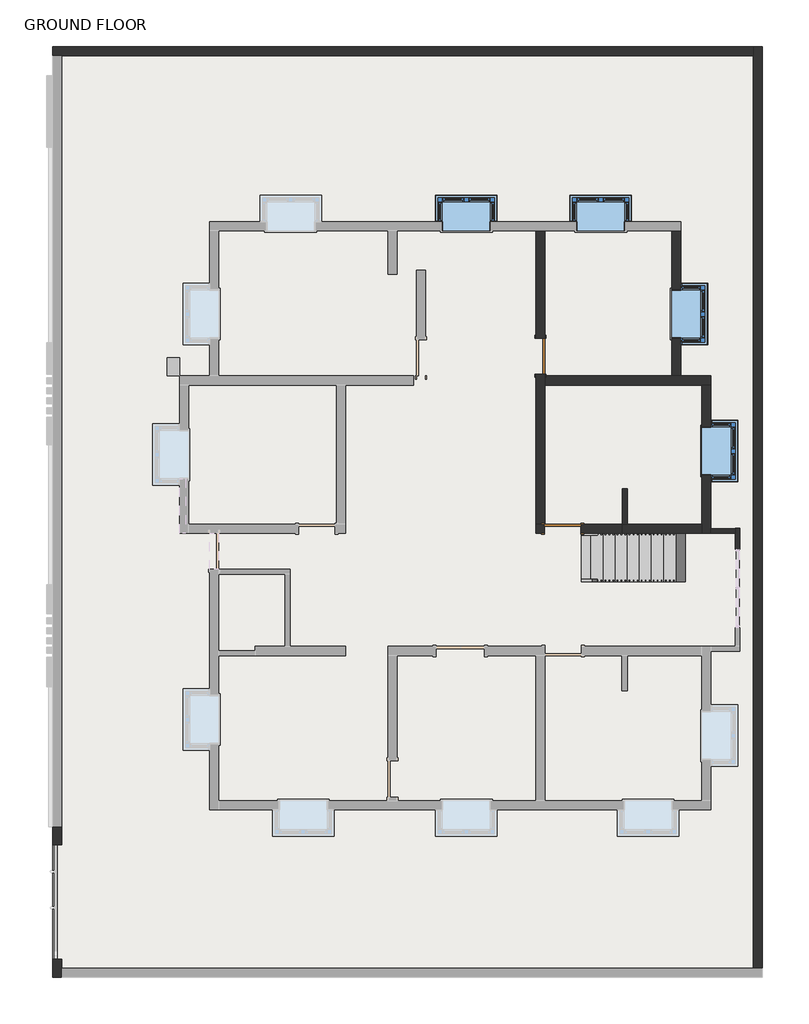
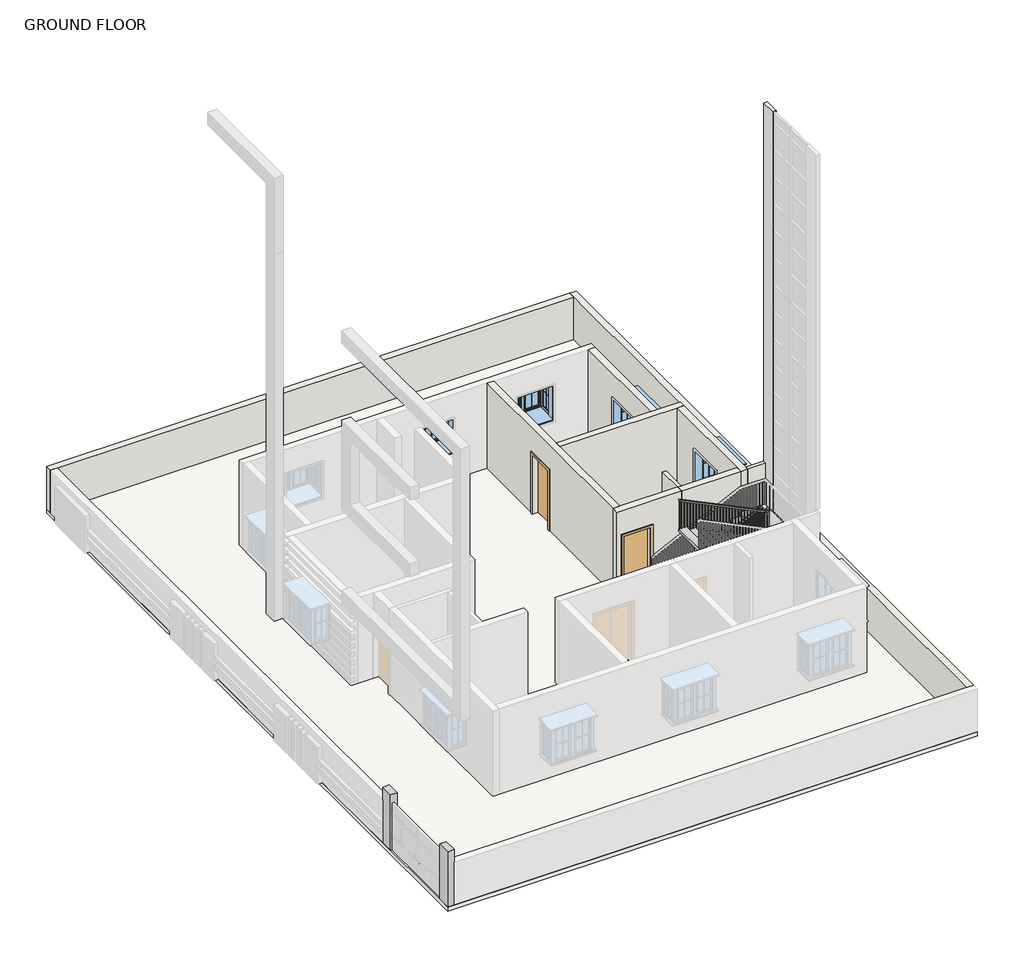
# One storey, part 3 of 5: 11 walls, 4 windows, 2 columns, 2 doors, 1 railing, 1 slab, 1 stair flight.
"""IFC4 building model written with IfcOpenShell, lengths in millimetres."""

from ifc_helpers import new_model, si_unit, frame, origin, origin_with_axes, place, context, project, spatial, polyline, outline, extrude, faceted_brep, transform, mapped, element, save
from components import door_a90ba1ad, door_0ca8825f, window_bay_casement_box_90_degree_angle_4_x4_x2_07b705a1

model = new_model("IFC4")

# Units and contexts
model_context = context("Model", 3, world=origin())
ifc_project = project(units=[si_unit("LENGTHUNIT", "METRE", prefix="MILLI")], contexts=[model_context])

# Site, building, storey
site = spatial("IfcSite", under=ifc_project)
building = spatial("IfcBuilding", under=site)
storey = spatial("IfcBuildingStorey", under=building, Name="GROUND FLOOR", Elevation=0.0)

# Columns
placement = place(None, origin())
element("IfcColumn", 1, ObjectType="Rectangular Column : 1.5' X9\"", at=placement, inside=storey, context=model_context, shape_type="Brep", body=[
    faceted_brep([(-10208.7415084, -10980.666654, 0.0), (-10208.7415084, -10523.466654, 0.0), (-9980.1415084, -10523.466654, 0.0), (-9980.1415084, -10752.066654, 0.0), (-9980.1415084, -10980.666654, 0.0), (-10208.7415084, -10980.666654, 1981.2), (-10208.7415084, -10523.466654, 1981.2), (-9980.1415084, -10523.466654, 1981.2), (-9980.1415084, -10980.666654, 1981.2), (-9980.1415084, -10980.666654, 1524.0)], [[[0, 1, 2, 3, 4]], [[5, 6, 1, 0]], [[6, 7, 2, 1]], [[7, 8, 9, 4, 3, 2]], [[8, 5, 0, 4, 9]], [[5, 8, 7, 6]]]),
])
element("IfcColumn", 2, ObjectType="Rectangular Column : 1.5' X9\"", at=placement, inside=storey, context=model_context, shape_type="Brep", body=[
    faceted_brep([(-10208.7415084, -7640.5661002, 0.0), (-10208.7415084, -7183.3661002, 0.0), (-9980.1415084, -7183.3661002, 0.0), (-9980.1415084, -7640.5661002, 0.0), (-10208.7415084, -7640.5661002, 1981.2), (-10208.7415084, -7183.3661002, 1981.2), (-10208.7415084, -7183.3661002, 1524.0), (-9980.1415084, -7183.3661002, 1981.2), (-9980.1415084, -7183.3661002, 1524.0), (-9980.1415084, -7640.5661002, 1981.2)], [[[0, 1, 2, 3]], [[4, 5, 6, 1, 0]], [[5, 7, 8, 2, 1, 6]], [[7, 9, 3, 2, 8]], [[9, 4, 0, 3]], [[4, 9, 7, 5]]]),
])

# Doors
door_shape = door_a90ba1ad(model_context)
element("IfcDoor", 3, ObjectType="Single-Flush : 36\" x 84\"", at=placement, inside=storey, context=model_context, shape_type="MappedRepresentation", body=[
    mapped(door_shape, transform((2656.3584916, 335.033346, 0.0), x_axis=(-1.0, 0.0, 0.0), y_axis=(0.0, -1.0, 0.0), z_axis=(0.0, 0.0, 1.0))),
])
door_2_shape = door_0ca8825f(model_context)
element("IfcDoor", 4, ObjectType="Single-Flush : 36\" x 84\"", at=placement, inside=storey, context=model_context, shape_type="MappedRepresentation", body=[
    mapped(door_2_shape, transform((2097.5584916, 4678.433346, 0.0), x_axis=(0.0, -1.0, 0.0), y_axis=(1.0, 0.0, 0.0), z_axis=(0.0, 0.0, 1.0))),
])

# Railing
element("IfcRailing", 5, ObjectType="Handrail - Rectangular", at=placement, inside=storey, context=model_context, shape_type="SolidModel", body=[
    faceted_brep([(3126.2584916, -947.666654, 1059.8727273), (3126.2584916, -947.666654, 1003.3956113), (3126.2584916, -998.466654, 1003.3956113), (3126.2584916, -998.466654, 1059.8727273), (6044.5829507, -947.666654, 2477.5823634), (6095.3829507, -947.666654, 2445.7836718), (6095.3829507, -998.466654, 2445.7836718), (6044.5829507, -998.466654, 2477.5823634), (6044.5829507, -947.666654, 2514.6), (6095.3829507, -947.666654, 2463.8), (6095.3829507, -998.466654, 2463.8), (6044.5829507, -998.466654, 2514.6), (6171.5829507, -947.666654, 2514.6), (6171.5829507, -947.666654, 2463.8), (6120.7829507, -998.466654, 2463.8), (6120.7829507, -998.466654, 2514.6), (6171.5829507, -1074.666654, 2514.6), (6171.5829507, -1074.666654, 2463.8), (6120.7829507, -1074.666654, 2463.8), (6120.7829507, -1074.666654, 2514.6), (6171.5829507, -1341.366654, 2514.6), (6171.5829507, -1392.166654, 2463.8), (6120.7829507, -1392.166654, 2463.8), (6120.7829507, -1341.366654, 2514.6), (6171.5829507, -1341.366654, 2697.0903639), (6171.5829507, -1392.166654, 2646.2903639), (6120.7829507, -1392.166654, 2646.2903639), (6120.7829507, -1341.366654, 2697.0903639), (6171.5829507, -1468.366654, 2697.0903639), (6171.5829507, -1468.366654, 2646.2903639), (6120.7829507, -1417.566654, 2646.2903639), (6120.7829507, -1417.566654, 2697.0903639), (6044.5829507, -1468.366654, 2697.0903639), (6032.8967309, -1468.366654, 2646.2903639), (6032.8967309, -1417.566654, 2646.2903639), (6044.5829507, -1417.566654, 2697.0903639), (3126.2584916, -1468.366654, 4114.8), (3126.2584916, -1417.566654, 4114.8), (3126.2584916, -1417.566654, 4058.322884), (3126.2584916, -1468.366654, 4058.322884)], [[[0, 1, 2, 3]], [[1, 0, 4, 5]], [[2, 1, 5, 6]], [[3, 2, 6, 7]], [[0, 3, 7, 4]], [[5, 4, 8, 9]], [[6, 5, 9, 10]], [[7, 6, 10, 11]], [[4, 7, 11, 8]], [[9, 8, 12, 13]], [[10, 9, 13, 14]], [[11, 10, 14, 15]], [[8, 11, 15, 12]], [[13, 12, 16, 17]], [[14, 13, 17, 18]], [[15, 14, 18, 19]], [[12, 15, 19, 16]], [[17, 16, 20, 21]], [[18, 17, 21, 22]], [[19, 18, 22, 23]], [[16, 19, 23, 20]], [[21, 20, 24, 25]], [[22, 21, 25, 26]], [[23, 22, 26, 27]], [[20, 23, 27, 24]], [[25, 24, 28, 29]], [[26, 25, 29, 30]], [[27, 26, 30, 31]], [[24, 27, 31, 28]], [[29, 28, 32, 33]], [[30, 29, 33, 34]], [[31, 30, 34, 35]], [[28, 31, 35, 32]], [[36, 37, 38, 39]], [[33, 32, 36, 39]], [[34, 33, 39, 38]], [[35, 34, 38, 37]], [[32, 35, 37, 36]]]),
    extrude(outline(polyline([(4017.9778093, 3209.3079507), (4027.2322184, 3190.2579507), (3054.9272727, 3190.2579507), (3054.9272727, 3209.3079507), (4017.9778093, 3209.3079507)])), frame((0.0, -1452.491654, 0.0), z_axis=(0.0, 1.0, 0.0), x_axis=(0.0, 0.0, 1.0)), (0.0, 0.0, 1.0), 19.05),
    extrude(outline(polyline([(3968.6209605, 3310.9079507), (3977.8753696, 3291.8579507), (3054.9272727, 3291.8579507), (3054.9272727, 3310.9079507), (3968.6209605, 3310.9079507)])), frame((0.0, -1452.491654, 0.0), z_axis=(0.0, 1.0, 0.0), x_axis=(0.0, 0.0, 1.0)), (0.0, 0.0, 1.0), 19.05),
    extrude(outline(polyline([(3919.2641117, 3412.5079507), (3928.5185208, 3393.4579507), (2909.4545455, 3393.4579507), (2909.4545455, 3412.5079507), (3919.2641117, 3412.5079507)])), frame((0.0, -1452.491654, 0.0), z_axis=(0.0, 1.0, 0.0), x_axis=(0.0, 0.0, 1.0)), (0.0, 0.0, 1.0), 19.05),
    extrude(outline(polyline([(3869.9072629, 3514.1079507), (3879.1616721, 3495.0579507), (2909.4545455, 3495.0579507), (2909.4545455, 3514.1079507), (3869.9072629, 3514.1079507)])), frame((0.0, -1452.491654, 0.0), z_axis=(0.0, 1.0, 0.0), x_axis=(0.0, 0.0, 1.0)), (0.0, 0.0, 1.0), 19.05),
    extrude(outline(polyline([(3820.5504141, 3615.7079507), (3829.8048233, 3596.6579507), (2909.4545455, 3596.6579507), (2909.4545455, 3615.7079507), (3820.5504141, 3615.7079507)])), frame((0.0, -1452.491654, 0.0), z_axis=(0.0, 1.0, 0.0), x_axis=(0.0, 0.0, 1.0)), (0.0, 0.0, 1.0), 19.05),
    extrude(outline(polyline([(3771.1935653, 3717.3079507), (3780.4479745, 3698.2579507), (2763.9818182, 3698.2579507), (2763.9818182, 3717.3079507), (3771.1935653, 3717.3079507)])), frame((0.0, -1452.491654, 0.0), z_axis=(0.0, 1.0, 0.0), x_axis=(0.0, 0.0, 1.0)), (0.0, 0.0, 1.0), 19.05),
    extrude(outline(polyline([(3721.8367166, 3818.9079507), (3731.0911257, 3799.8579507), (2763.9818182, 3799.8579507), (2763.9818182, 3818.9079507), (3721.8367166, 3818.9079507)])), frame((0.0, -1452.491654, 0.0), z_axis=(0.0, 1.0, 0.0), x_axis=(0.0, 0.0, 1.0)), (0.0, 0.0, 1.0), 19.05),
    extrude(outline(polyline([(3672.4798678, 3920.5079507), (3681.7342769, 3901.4579507), (2763.9818182, 3901.4579507), (2763.9818182, 3920.5079507), (3672.4798678, 3920.5079507)])), frame((0.0, -1452.491654, 0.0), z_axis=(0.0, 1.0, 0.0), x_axis=(0.0, 0.0, 1.0)), (0.0, 0.0, 1.0), 19.05),
    extrude(outline(polyline([(3623.123019, 4022.1079507), (3632.3774281, 4003.0579507), (2618.5090909, 4003.0579507), (2618.5090909, 4022.1079507), (3623.123019, 4022.1079507)])), frame((0.0, -1452.491654, 0.0), z_axis=(0.0, 1.0, 0.0), x_axis=(0.0, 0.0, 1.0)), (0.0, 0.0, 1.0), 19.05),
    extrude(outline(polyline([(3573.7661702, 4123.7079507), (3583.0205793, 4104.6579507), (2618.5090909, 4104.6579507), (2618.5090909, 4123.7079507), (3573.7661702, 4123.7079507)])), frame((0.0, -1452.491654, 0.0), z_axis=(0.0, 1.0, 0.0), x_axis=(0.0, 0.0, 1.0)), (0.0, 0.0, 1.0), 19.05),
    extrude(outline(polyline([(3524.4093214, 4225.3079507), (3533.6637306, 4206.2579507), (2618.5090909, 4206.2579507), (2618.5090909, 4225.3079507), (3524.4093214, 4225.3079507)])), frame((0.0, -1452.491654, 0.0), z_axis=(0.0, 1.0, 0.0), x_axis=(0.0, 0.0, 1.0)), (0.0, 0.0, 1.0), 19.05),
    extrude(outline(polyline([(3475.0524726, 4326.9079507), (3484.3068818, 4307.8579507), (2473.0363636, 4307.8579507), (2473.0363636, 4326.9079507), (3475.0524726, 4326.9079507)])), frame((0.0, -1452.491654, 0.0), z_axis=(0.0, 1.0, 0.0), x_axis=(0.0, 0.0, 1.0)), (0.0, 0.0, 1.0), 19.05),
    extrude(outline(polyline([(3425.6956238, 4428.5079507), (3434.950033, 4409.4579507), (2473.0363636, 4409.4579507), (2473.0363636, 4428.5079507), (3425.6956238, 4428.5079507)])), frame((0.0, -1452.491654, 0.0), z_axis=(0.0, 1.0, 0.0), x_axis=(0.0, 0.0, 1.0)), (0.0, 0.0, 1.0), 19.05),
    extrude(outline(polyline([(3376.3387751, 4530.1079507), (3385.5931842, 4511.0579507), (2473.0363636, 4511.0579507), (2473.0363636, 4530.1079507), (3376.3387751, 4530.1079507)])), frame((0.0, -1452.491654, 0.0), z_axis=(0.0, 1.0, 0.0), x_axis=(0.0, 0.0, 1.0)), (0.0, 0.0, 1.0), 19.05),
    extrude(outline(polyline([(3326.9819263, 4631.7079507), (3336.2363354, 4612.6579507), (2327.5636364, 4612.6579507), (2327.5636364, 4631.7079507), (3326.9819263, 4631.7079507)])), frame((0.0, -1452.491654, 0.0), z_axis=(0.0, 1.0, 0.0), x_axis=(0.0, 0.0, 1.0)), (0.0, 0.0, 1.0), 19.05),
    extrude(outline(polyline([(3277.6250775, 4733.3079507), (3286.8794866, 4714.2579507), (2327.5636364, 4714.2579507), (2327.5636364, 4733.3079507), (3277.6250775, 4733.3079507)])), frame((0.0, -1452.491654, 0.0), z_axis=(0.0, 1.0, 0.0), x_axis=(0.0, 0.0, 1.0)), (0.0, 0.0, 1.0), 19.05),
    extrude(outline(polyline([(3228.2682287, 4834.9079507), (3237.5226379, 4815.8579507), (2327.5636364, 4815.8579507), (2327.5636364, 4834.9079507), (3228.2682287, 4834.9079507)])), frame((0.0, -1452.491654, 0.0), z_axis=(0.0, 1.0, 0.0), x_axis=(0.0, 0.0, 1.0)), (0.0, 0.0, 1.0), 19.05),
    extrude(outline(polyline([(3178.9113799, 4936.5079507), (3188.1657891, 4917.4579507), (2182.0909091, 4917.4579507), (2182.0909091, 4936.5079507), (3178.9113799, 4936.5079507)])), frame((0.0, -1452.491654, 0.0), z_axis=(0.0, 1.0, 0.0), x_axis=(0.0, 0.0, 1.0)), (0.0, 0.0, 1.0), 19.05),
    extrude(outline(polyline([(3129.5545311, 5038.1079507), (3138.8089403, 5019.0579507), (2182.0909091, 5019.0579507), (2182.0909091, 5038.1079507), (3129.5545311, 5038.1079507)])), frame((0.0, -1452.491654, 0.0), z_axis=(0.0, 1.0, 0.0), x_axis=(0.0, 0.0, 1.0)), (0.0, 0.0, 1.0), 19.05),
    extrude(outline(polyline([(3080.1976824, 5139.7079507), (3089.4520915, 5120.6579507), (2182.0909091, 5120.6579507), (2182.0909091, 5139.7079507), (3080.1976824, 5139.7079507)])), frame((0.0, -1452.491654, 0.0), z_axis=(0.0, 1.0, 0.0), x_axis=(0.0, 0.0, 1.0)), (0.0, 0.0, 1.0), 19.05),
    extrude(outline(polyline([(3030.759384, 5241.3079507), (3040.0137931, 5222.2579507), (2036.6181818, 5222.2579507), (2036.6181818, 5241.3079507), (3030.759384, 5241.3079507)])), frame((0.0, -1452.491654, 0.0), z_axis=(0.0, 1.0, 0.0), x_axis=(0.0, 0.0, 1.0)), (0.0, 0.0, 1.0), 19.05),
    extrude(outline(polyline([(2981.4839848, 5342.9079507), (2990.7383939, 5323.8579507), (2036.6181818, 5323.8579507), (2036.6181818, 5342.9079507), (2981.4839848, 5342.9079507)])), frame((0.0, -1452.491654, 0.0), z_axis=(0.0, 1.0, 0.0), x_axis=(0.0, 0.0, 1.0)), (0.0, 0.0, 1.0), 19.05),
    extrude(outline(polyline([(2932.127136, 5444.5079507), (2941.3815452, 5425.4579507), (2036.6181818, 5425.4579507), (2036.6181818, 5444.5079507), (2932.127136, 5444.5079507)])), frame((0.0, -1452.491654, 0.0), z_axis=(0.0, 1.0, 0.0), x_axis=(0.0, 0.0, 1.0)), (0.0, 0.0, 1.0), 19.05),
    extrude(outline(polyline([(2882.7702872, 5546.1079507), (2892.0246964, 5527.0579507), (1891.1454545, 5527.0579507), (1891.1454545, 5546.1079507), (2882.7702872, 5546.1079507)])), frame((0.0, -1452.491654, 0.0), z_axis=(0.0, 1.0, 0.0), x_axis=(0.0, 0.0, 1.0)), (0.0, 0.0, 1.0), 19.05),
    extrude(outline(polyline([(2833.4134384, 5647.7079507), (2842.6678476, 5628.6579507), (1891.1454545, 5628.6579507), (1891.1454545, 5647.7079507), (2833.4134384, 5647.7079507)])), frame((0.0, -1452.491654, 0.0), z_axis=(0.0, 1.0, 0.0), x_axis=(0.0, 0.0, 1.0)), (0.0, 0.0, 1.0), 19.05),
    extrude(outline(polyline([(2784.0565897, 5749.3079507), (2793.3109988, 5730.2579507), (1891.1454545, 5730.2579507), (1891.1454545, 5749.3079507), (2784.0565897, 5749.3079507)])), frame((0.0, -1452.491654, 0.0), z_axis=(0.0, 1.0, 0.0), x_axis=(0.0, 0.0, 1.0)), (0.0, 0.0, 1.0), 19.05),
    extrude(outline(polyline([(2734.6997409, 5850.9079507), (2743.95415, 5831.8579507), (1745.6727273, 5831.8579507), (1745.6727273, 5850.9079507), (2734.6997409, 5850.9079507)])), frame((0.0, -1452.491654, 0.0), z_axis=(0.0, 1.0, 0.0), x_axis=(0.0, 0.0, 1.0)), (0.0, 0.0, 1.0), 19.05),
    extrude(outline(polyline([(2685.3428921, 5952.5079507), (2694.5973012, 5933.4579507), (1745.6727273, 5933.4579507), (1745.6727273, 5952.5079507), (2685.3428921, 5952.5079507)])), frame((0.0, -1452.491654, 0.0), z_axis=(0.0, 1.0, 0.0), x_axis=(0.0, 0.0, 1.0)), (0.0, 0.0, 1.0), 19.05),
    extrude(outline(polyline([(2635.9860433, 6054.1079507), (2645.2404524, 6035.0579507), (1745.6727273, 6035.0579507), (1745.6727273, 6054.1079507), (2635.9860433, 6054.1079507)])), frame((0.0, -1452.491654, 0.0), z_axis=(0.0, 1.0, 0.0), x_axis=(0.0, 0.0, 1.0)), (0.0, 0.0, 1.0), 19.05),
    extrude(outline(polyline([(6136.6579507, -1369.941654), (6155.7079507, -1369.941654), (6155.7079507, -1388.991654), (6136.6579507, -1388.991654), (6136.6579507, -1369.941654)])), frame((0.0, 0.0, 1600.2), z_axis=(0.0, 0.0, 1.0), x_axis=(1.0, 0.0, 0.0)), (0.0, 0.0, 1.0), 1046.0903639),
    extrude(outline(polyline([(6136.6579507, -1268.341654), (6155.7079507, -1268.341654), (6155.7079507, -1287.391654), (6136.6579507, -1287.391654), (6136.6579507, -1268.341654)])), frame((0.0, 0.0, 1600.2), z_axis=(0.0, 0.0, 1.0), x_axis=(1.0, 0.0, 0.0)), (0.0, 0.0, 1.0), 863.6),
    extrude(outline(polyline([(6136.6579507, -1166.741654), (6155.7079507, -1166.741654), (6155.7079507, -1185.791654), (6136.6579507, -1185.791654), (6136.6579507, -1166.741654)])), frame((0.0, 0.0, 1600.2), z_axis=(0.0, 0.0, 1.0), x_axis=(1.0, 0.0, 0.0)), (0.0, 0.0, 1.0), 863.6),
    extrude(outline(polyline([(6136.6579507, -1065.141654), (6155.7079507, -1065.141654), (6155.7079507, -1084.191654), (6136.6579507, -1084.191654), (6136.6579507, -1065.141654)])), frame((0.0, 0.0, 1600.2), z_axis=(0.0, 0.0, 1.0), x_axis=(1.0, 0.0, 0.0)), (0.0, 0.0, 1.0), 863.6),
    extrude(outline(polyline([(6063.1334916, -982.591654), (6063.1334916, -963.541654), (6082.1834916, -963.541654), (6082.1834916, -982.591654), (6063.1334916, -982.591654)])), frame((0.0, 0.0, 1454.7272727), z_axis=(0.0, 0.0, 1.0), x_axis=(1.0, 0.0, 0.0)), (0.0, 0.0, 1.0), 1009.0727273),
    extrude(outline(polyline([(2390.0145818, 5980.5834916), (2380.7601727, 5961.5334916), (1454.7272727, 5961.5334916), (1454.7272727, 5980.5834916), (2390.0145818, 5980.5834916)])), frame((0.0, -982.591654, 0.0), z_axis=(0.0, 1.0, 0.0), x_axis=(0.0, 0.0, 1.0)), (0.0, 0.0, 1.0), 19.05),
    extrude(outline(polyline([(2340.657733, 5878.9834916), (2331.4033239, 5859.9334916), (1454.7272727, 5859.9334916), (1454.7272727, 5878.9834916), (2340.657733, 5878.9834916)])), frame((0.0, -982.591654, 0.0), z_axis=(0.0, 1.0, 0.0), x_axis=(0.0, 0.0, 1.0)), (0.0, 0.0, 1.0), 19.05),
    extrude(outline(polyline([(2291.3008843, 5777.3834916), (2282.0464751, 5758.3334916), (1309.2545455, 5758.3334916), (1309.2545455, 5777.3834916), (2291.3008843, 5777.3834916)])), frame((0.0, -982.591654, 0.0), z_axis=(0.0, 1.0, 0.0), x_axis=(0.0, 0.0, 1.0)), (0.0, 0.0, 1.0), 19.05),
    extrude(outline(polyline([(2241.9440355, 5675.7834916), (2232.6896263, 5656.7334916), (1309.2545455, 5656.7334916), (1309.2545455, 5675.7834916), (2241.9440355, 5675.7834916)])), frame((0.0, -982.591654, 0.0), z_axis=(0.0, 1.0, 0.0), x_axis=(0.0, 0.0, 1.0)), (0.0, 0.0, 1.0), 19.05),
    extrude(outline(polyline([(2192.5871867, 5574.1834916), (2183.3327775, 5555.1334916), (1309.2545455, 5555.1334916), (1309.2545455, 5574.1834916), (2192.5871867, 5574.1834916)])), frame((0.0, -982.591654, 0.0), z_axis=(0.0, 1.0, 0.0), x_axis=(0.0, 0.0, 1.0)), (0.0, 0.0, 1.0), 19.05),
    extrude(outline(polyline([(2143.2303379, 5472.5834916), (2133.9759288, 5453.5334916), (1163.7818182, 5453.5334916), (1163.7818182, 5472.5834916), (2143.2303379, 5472.5834916)])), frame((0.0, -982.591654, 0.0), z_axis=(0.0, 1.0, 0.0), x_axis=(0.0, 0.0, 1.0)), (0.0, 0.0, 1.0), 19.05),
    extrude(outline(polyline([(2093.8734891, 5370.9834916), (2084.61908, 5351.9334916), (1163.7818182, 5351.9334916), (1163.7818182, 5370.9834916), (2093.8734891, 5370.9834916)])), frame((0.0, -982.591654, 0.0), z_axis=(0.0, 1.0, 0.0), x_axis=(0.0, 0.0, 1.0)), (0.0, 0.0, 1.0), 19.05),
    extrude(outline(polyline([(2044.5166403, 5269.3834916), (2035.2622312, 5250.3334916), (1163.7818182, 5250.3334916), (1163.7818182, 5269.3834916), (2044.5166403, 5269.3834916)])), frame((0.0, -982.591654, 0.0), z_axis=(0.0, 1.0, 0.0), x_axis=(0.0, 0.0, 1.0)), (0.0, 0.0, 1.0), 19.05),
    extrude(outline(polyline([(1995.1597915, 5167.7834916), (1985.9053824, 5148.7334916), (1018.3090909, 5148.7334916), (1018.3090909, 5167.7834916), (1995.1597915, 5167.7834916)])), frame((0.0, -982.591654, 0.0), z_axis=(0.0, 1.0, 0.0), x_axis=(0.0, 0.0, 1.0)), (0.0, 0.0, 1.0), 19.05),
    extrude(outline(polyline([(1945.8029428, 5066.1834916), (1936.5485336, 5047.1334916), (1018.3090909, 5047.1334916), (1018.3090909, 5066.1834916), (1945.8029428, 5066.1834916)])), frame((0.0, -982.591654, 0.0), z_axis=(0.0, 1.0, 0.0), x_axis=(0.0, 0.0, 1.0)), (0.0, 0.0, 1.0), 19.05),
    extrude(outline(polyline([(1896.446094, 4964.5834916), (1887.1916848, 4945.5334916), (1018.3090909, 4945.5334916), (1018.3090909, 4964.5834916), (1896.446094, 4964.5834916)])), frame((0.0, -982.591654, 0.0), z_axis=(0.0, 1.0, 0.0), x_axis=(0.0, 0.0, 1.0)), (0.0, 0.0, 1.0), 19.05),
    extrude(outline(polyline([(1847.0892452, 4862.9834916), (1837.834836, 4843.9334916), (872.8363636, 4843.9334916), (872.8363636, 4862.9834916), (1847.0892452, 4862.9834916)])), frame((0.0, -982.591654, 0.0), z_axis=(0.0, 1.0, 0.0), x_axis=(0.0, 0.0, 1.0)), (0.0, 0.0, 1.0), 19.05),
    extrude(outline(polyline([(1797.7323964, 4761.3834916), (1788.4779873, 4742.3334916), (872.8363636, 4742.3334916), (872.8363636, 4761.3834916), (1797.7323964, 4761.3834916)])), frame((0.0, -982.591654, 0.0), z_axis=(0.0, 1.0, 0.0), x_axis=(0.0, 0.0, 1.0)), (0.0, 0.0, 1.0), 19.05),
    extrude(outline(polyline([(1748.3755476, 4659.7834916), (1739.1211385, 4640.7334916), (872.8363636, 4640.7334916), (872.8363636, 4659.7834916), (1748.3755476, 4659.7834916)])), frame((0.0, -982.591654, 0.0), z_axis=(0.0, 1.0, 0.0), x_axis=(0.0, 0.0, 1.0)), (0.0, 0.0, 1.0), 19.05),
    extrude(outline(polyline([(1699.0186988, 4558.1834916), (1689.7642897, 4539.1334916), (727.3636364, 4539.1334916), (727.3636364, 4558.1834916), (1699.0186988, 4558.1834916)])), frame((0.0, -982.591654, 0.0), z_axis=(0.0, 1.0, 0.0), x_axis=(0.0, 0.0, 1.0)), (0.0, 0.0, 1.0), 19.05),
    extrude(outline(polyline([(1649.6618501, 4456.5834916), (1640.4074409, 4437.5334916), (727.3636364, 4437.5334916), (727.3636364, 4456.5834916), (1649.6618501, 4456.5834916)])), frame((0.0, -982.591654, 0.0), z_axis=(0.0, 1.0, 0.0), x_axis=(0.0, 0.0, 1.0)), (0.0, 0.0, 1.0), 19.05),
    extrude(outline(polyline([(1600.3050013, 4354.9834916), (1591.0505921, 4335.9334916), (727.3636364, 4335.9334916), (727.3636364, 4354.9834916), (1600.3050013, 4354.9834916)])), frame((0.0, -982.591654, 0.0), z_axis=(0.0, 1.0, 0.0), x_axis=(0.0, 0.0, 1.0)), (0.0, 0.0, 1.0), 19.05),
    extrude(outline(polyline([(1550.9481525, 4253.3834916), (1541.6937433, 4234.3334916), (581.8909091, 4234.3334916), (581.8909091, 4253.3834916), (1550.9481525, 4253.3834916)])), frame((0.0, -982.591654, 0.0), z_axis=(0.0, 1.0, 0.0), x_axis=(0.0, 0.0, 1.0)), (0.0, 0.0, 1.0), 19.05),
    extrude(outline(polyline([(1501.5913037, 4151.7834916), (1492.3368946, 4132.7334916), (581.8909091, 4132.7334916), (581.8909091, 4151.7834916), (1501.5913037, 4151.7834916)])), frame((0.0, -982.591654, 0.0), z_axis=(0.0, 1.0, 0.0), x_axis=(0.0, 0.0, 1.0)), (0.0, 0.0, 1.0), 19.05),
    extrude(outline(polyline([(1452.2344549, 4050.1834916), (1442.9800458, 4031.1334916), (581.8909091, 4031.1334916), (581.8909091, 4050.1834916), (1452.2344549, 4050.1834916)])), frame((0.0, -982.591654, 0.0), z_axis=(0.0, 1.0, 0.0), x_axis=(0.0, 0.0, 1.0)), (0.0, 0.0, 1.0), 19.05),
    extrude(outline(polyline([(1402.8776061, 3948.5834916), (1393.623197, 3929.5334916), (436.4181818, 3929.5334916), (436.4181818, 3948.5834916), (1402.8776061, 3948.5834916)])), frame((0.0, -982.591654, 0.0), z_axis=(0.0, 1.0, 0.0), x_axis=(0.0, 0.0, 1.0)), (0.0, 0.0, 1.0), 19.05),
    extrude(outline(polyline([(1353.5207573, 3846.9834916), (1344.2663482, 3827.9334916), (436.4181818, 3827.9334916), (436.4181818, 3846.9834916), (1353.5207573, 3846.9834916)])), frame((0.0, -982.591654, 0.0), z_axis=(0.0, 1.0, 0.0), x_axis=(0.0, 0.0, 1.0)), (0.0, 0.0, 1.0), 19.05),
    extrude(outline(polyline([(1304.1639086, 3745.3834916), (1294.9094994, 3726.3334916), (436.4181818, 3726.3334916), (436.4181818, 3745.3834916), (1304.1639086, 3745.3834916)])), frame((0.0, -982.591654, 0.0), z_axis=(0.0, 1.0, 0.0), x_axis=(0.0, 0.0, 1.0)), (0.0, 0.0, 1.0), 19.05),
    extrude(outline(polyline([(1254.8070598, 3643.7834916), (1245.5526506, 3624.7334916), (290.9454545, 3624.7334916), (290.9454545, 3643.7834916), (1254.8070598, 3643.7834916)])), frame((0.0, -982.591654, 0.0), z_axis=(0.0, 1.0, 0.0), x_axis=(0.0, 0.0, 1.0)), (0.0, 0.0, 1.0), 19.05),
    extrude(outline(polyline([(1205.450211, 3542.1834916), (1196.1958018, 3523.1334916), (290.9454545, 3523.1334916), (290.9454545, 3542.1834916), (1205.450211, 3542.1834916)])), frame((0.0, -982.591654, 0.0), z_axis=(0.0, 1.0, 0.0), x_axis=(0.0, 0.0, 1.0)), (0.0, 0.0, 1.0), 19.05),
    extrude(outline(polyline([(1156.0933622, 3440.5834916), (1146.8389531, 3421.5334916), (290.9454545, 3421.5334916), (290.9454545, 3440.5834916), (1156.0933622, 3440.5834916)])), frame((0.0, -982.591654, 0.0), z_axis=(0.0, 1.0, 0.0), x_axis=(0.0, 0.0, 1.0)), (0.0, 0.0, 1.0), 19.05),
    extrude(outline(polyline([(1106.7365134, 3338.9834916), (1097.4821043, 3319.9334916), (145.4727273, 3319.9334916), (145.4727273, 3338.9834916), (1106.7365134, 3338.9834916)])), frame((0.0, -982.591654, 0.0), z_axis=(0.0, 1.0, 0.0), x_axis=(0.0, 0.0, 1.0)), (0.0, 0.0, 1.0), 19.05),
    extrude(outline(polyline([(1057.3796646, 3237.3834916), (1048.1252555, 3218.3334916), (145.4727273, 3218.3334916), (145.4727273, 3237.3834916), (1057.3796646, 3237.3834916)])), frame((0.0, -982.591654, 0.0), z_axis=(0.0, 1.0, 0.0), x_axis=(0.0, 0.0, 1.0)), (0.0, 0.0, 1.0), 19.05),
    extrude(outline(polyline([(6136.6579507, -1433.441654), (6155.7079507, -1433.441654), (6155.7079507, -1452.491654), (6136.6579507, -1452.491654), (6136.6579507, -1433.441654)])), frame((0.0, 0.0, 1600.2), z_axis=(0.0, 0.0, 1.0), x_axis=(1.0, 0.0, 0.0)), (0.0, 0.0, 1.0), 1046.0903639),
    extrude(outline(polyline([(6136.6579507, -982.591654), (6136.6579507, -963.541654), (6155.7079507, -963.541654), (6155.7079507, -982.591654), (6136.6579507, -982.591654)])), frame((0.0, 0.0, 1600.2), z_axis=(0.0, 0.0, 1.0), x_axis=(1.0, 0.0, 0.0)), (0.0, 0.0, 1.0), 863.6),
    extrude(outline(polyline([(4049.0684749, 3145.3084916), (4058.322884, 3126.2584916), (3054.9272727, 3126.2584916), (3054.9272727, 3145.3084916), (4049.0684749, 3145.3084916)])), frame((0.0, -1452.491654, 0.0), z_axis=(0.0, 1.0, 0.0), x_axis=(0.0, 0.0, 1.0)), (0.0, 0.0, 1.0), 19.05),
    extrude(outline(polyline([(1012.6500204, 3145.3084916), (1003.3956113, 3126.2584916), (145.4727273, 3126.2584916), (145.4727273, 3145.3084916), (1012.6500204, 3145.3084916)])), frame((0.0, -982.591654, 0.0), z_axis=(0.0, 1.0, 0.0), x_axis=(0.0, 0.0, 1.0)), (0.0, 0.0, 1.0), 19.05),
])

# Slab
element("IfcSlab", 6, ObjectType="6\"", at=placement, inside=storey, context=model_context, shape_type="SweptSolid", body=[
    extrude(outline(polyline([(7698.2584916, 12488.933346), (7698.2584916, -10980.666654), (-10208.7415084, -10980.666654), (-10208.7415084, 12488.933346), (7698.2584916, 12488.933346)])), frame((0.0, 0.0, -152.4), z_axis=(0.0, 0.0, 1.0), x_axis=(1.0, 0.0, 0.0)), (0.0, 0.0, 1.0), 152.4),
])

# Stair flight
element("IfcStairFlight", 7, ObjectType="3/4\" Nosing", at=placement, inside=storey, context=model_context, shape_type="Brep", body=[
    faceted_brep([(3126.2584916, 220.733346, 145.4727273), (3126.2584916, -998.466654, 145.4727273), (3396.6329507, -998.466654, 145.4727273), (3396.6329507, 220.733346, 145.4727273), (3396.6329507, 220.733346, 81.9727273), (3134.5739678, 220.733346, 81.9727273), (3134.5739678, -998.466654, 81.9727273), (3396.6329507, -998.466654, 81.9727273), (3377.5829507, 220.733346, 290.9454545), (3377.5829507, -998.466654, 290.9454545), (3411.0096137, -998.466654, 290.9454545), (3701.4329507, -998.466654, 290.9454545), (3701.4329507, 220.733346, 290.9454545), (3411.0096137, 220.733346, 290.9454545), (3701.4329507, 220.733346, 220.5838654), (3411.0096137, 220.733346, 81.9727273), (3411.0096137, -998.466654, 81.9727273), (3701.4329507, -998.466654, 220.5838654), (3682.3829507, 220.733346, 436.4181818), (3682.3829507, -998.466654, 436.4181818), (4006.2329507, -998.466654, 436.4181818), (4006.2329507, 220.733346, 436.4181818), (4006.2329507, 220.733346, 366.0565927), (4006.2329507, -998.466654, 366.0565927), (3987.1829507, 220.733346, 581.8909091), (3987.1829507, -998.466654, 581.8909091), (4311.0329507, -998.466654, 581.8909091), (4311.0329507, 220.733346, 581.8909091), (4311.0329507, 220.733346, 511.5293199), (4311.0329507, -998.466654, 511.5293199), (4291.9829507, 220.733346, 727.3636364), (4291.9829507, -998.466654, 727.3636364), (4615.8329507, -998.466654, 727.3636364), (4615.8329507, 220.733346, 727.3636364), (4615.8329507, 220.733346, 657.0020472), (4615.8329507, -998.466654, 657.0020472), (4596.7829507, 220.733346, 872.8363636), (4596.7829507, -998.466654, 872.8363636), (4920.6329507, -998.466654, 872.8363636), (4920.6329507, 220.733346, 872.8363636), (4920.6329507, 220.733346, 802.4747745), (4920.6329507, -998.466654, 802.4747745), (4901.5829507, 220.733346, 1018.3090909), (4901.5829507, -998.466654, 1018.3090909), (5225.4329507, -998.466654, 1018.3090909), (5225.4329507, 220.733346, 1018.3090909), (5225.4329507, 220.733346, 947.9475018), (5225.4329507, -998.466654, 947.9475018), (5206.3829507, 220.733346, 1163.7818182), (5206.3829507, -998.466654, 1163.7818182), (5530.2329507, -998.466654, 1163.7818182), (5530.2329507, 220.733346, 1163.7818182), (5530.2329507, 220.733346, 1093.420229), (5530.2329507, -998.466654, 1093.420229), (5511.1829507, 220.733346, 1309.2545455), (5511.1829507, -998.466654, 1309.2545455), (5835.0329507, -998.466654, 1309.2545455), (5835.0329507, 220.733346, 1309.2545455), (5835.0329507, 220.733346, 1238.8929563), (5835.0329507, -998.466654, 1238.8929563), (5815.9829507, 220.733346, 1454.7272727), (5815.9829507, -998.466654, 1454.7272727), (6139.8329507, -998.466654, 1454.7272727), (6139.8329507, 220.733346, 1454.7272727), (6139.8329507, 220.733346, 1384.3656836), (6459.0096137, -998.466654, 1536.7), (6129.0984269, -998.466654, 1536.7), (6101.7329507, -2636.766654, 1600.2), (7009.1350459, -2636.766654, 1600.2), (7009.1350459, 220.733346, 1600.2), (6459.0096137, 220.733346, 1600.2), (6120.7829507, 220.733346, 1600.2), (6120.7829507, -998.466654, 1600.2), (6120.7829507, -1417.566654, 1600.2), (6101.7329507, -1417.566654, 1600.2), (6101.7329507, -2636.766654, 1536.7), (7009.1350459, -2636.766654, 1536.7), (7009.1350459, 220.733346, 1536.7), (6459.0096137, 220.733346, 1536.7), (6120.7829507, -998.466654, 1536.7), (6120.7829507, -1417.566654, 1536.7), (6101.7329507, -1417.566654, 1536.7), (6120.7829507, -2636.766654, 1745.6727273), (6120.7829507, -1417.566654, 1745.6727273), (6087.3562877, -1417.566654, 1745.6727273), (5796.9329507, -1417.566654, 1745.6727273), (5796.9329507, -2636.766654, 1745.6727273), (6087.3562877, -2636.766654, 1745.6727273), (5796.9329507, -2636.766654, 1675.3111381), (6087.3562877, -2636.766654, 1536.7), (6087.3562877, -1417.566654, 1536.7), (5796.9329507, -1417.566654, 1675.3111381), (5815.9829507, -2636.766654, 1891.1454545), (5815.9829507, -1417.566654, 1891.1454545), (5492.1329507, -1417.566654, 1891.1454545), (5492.1329507, -2636.766654, 1891.1454545), (5492.1329507, -2636.766654, 1820.7838654), (5492.1329507, -1417.566654, 1820.7838654), (5511.1829507, -2636.766654, 2036.6181818), (5511.1829507, -1417.566654, 2036.6181818), (5187.3329507, -1417.566654, 2036.6181818), (5187.3329507, -2636.766654, 2036.6181818), (5187.3329507, -2636.766654, 1966.2565927), (5187.3329507, -1417.566654, 1966.2565927), (5206.3829507, -2636.766654, 2182.0909091), (5206.3829507, -1417.566654, 2182.0909091), (4882.5329507, -1417.566654, 2182.0909091), (4882.5329507, -2636.766654, 2182.0909091), (4882.5329507, -2636.766654, 2111.7293199), (4882.5329507, -1417.566654, 2111.7293199), (4901.5829507, -2636.766654, 2327.5636364), (4901.5829507, -1417.566654, 2327.5636364), (4577.7329507, -1417.566654, 2327.5636364), (4577.7329507, -2636.766654, 2327.5636364), (4577.7329507, -2636.766654, 2257.2020472), (4577.7329507, -1417.566654, 2257.2020472), (4596.7829507, -2636.766654, 2473.0363636), (4596.7829507, -1417.566654, 2473.0363636), (4272.9329507, -1417.566654, 2473.0363636), (4272.9329507, -2636.766654, 2473.0363636), (4272.9329507, -2636.766654, 2402.6747745), (4272.9329507, -1417.566654, 2402.6747745), (4291.9829507, -2636.766654, 2618.5090909), (4291.9829507, -1417.566654, 2618.5090909), (3968.1329507, -1417.566654, 2618.5090909), (3968.1329507, -2636.766654, 2618.5090909), (3968.1329507, -2636.766654, 2548.1475018), (3968.1329507, -1417.566654, 2548.1475018), (3987.1829507, -2636.766654, 2763.9818182), (3987.1829507, -1417.566654, 2763.9818182), (3663.3329507, -1417.566654, 2763.9818182), (3663.3329507, -2636.766654, 2763.9818182), (3663.3329507, -2636.766654, 2693.620229), (3663.3329507, -1417.566654, 2693.620229), (3682.3829507, -2636.766654, 2909.4545455), (3682.3829507, -1417.566654, 2909.4545455), (3358.5329507, -1417.566654, 2909.4545455), (3358.5329507, -2636.766654, 2909.4545455), (3358.5329507, -2636.766654, 2839.0929563), (3358.5329507, -1417.566654, 2839.0929563), (3377.5829507, -2636.766654, 3054.9272727), (3377.5829507, -1417.566654, 3054.9272727), (3126.2584916, -1417.566654, 3054.9272727), (3126.2584916, -2636.766654, 3054.9272727), (3126.2584916, -2636.766654, 2949.9512209), (3126.2584916, -1417.566654, 2949.9512209)], [[[0, 1, 2, 3]], [[0, 3, 4, 5]], [[2, 1, 6, 7]], [[8, 9, 10, 11, 12, 13]], [[3, 8, 13, 12, 14, 15, 4]], [[9, 2, 7, 16, 17, 11, 10]], [[18, 19, 20, 21]], [[18, 21, 22, 14, 12]], [[20, 19, 11, 17, 23]], [[24, 25, 26, 27]], [[24, 27, 28, 22, 21]], [[26, 25, 20, 23, 29]], [[30, 31, 32, 33]], [[30, 33, 34, 28, 27]], [[32, 31, 26, 29, 35]], [[36, 37, 38, 39]], [[36, 39, 40, 34, 33]], [[38, 37, 32, 35, 41]], [[42, 43, 44, 45]], [[42, 45, 46, 40, 39]], [[44, 43, 38, 41, 47]], [[48, 49, 50, 51]], [[48, 51, 52, 46, 45]], [[50, 49, 44, 47, 53]], [[54, 55, 56, 57]], [[54, 57, 58, 52, 51]], [[56, 55, 50, 53, 59]], [[60, 61, 62, 63]], [[60, 63, 64, 58, 57]], [[61, 56, 59, 65, 66, 62]], [[67, 68, 69, 70, 71, 72, 73, 74]], [[68, 67, 75, 76]], [[69, 68, 76, 77]], [[63, 71, 70, 69, 77, 78, 64]], [[72, 66, 79]], [[73, 72, 79, 80]], [[74, 73, 80, 81]], [[82, 83, 84, 85, 86, 87]], [[67, 82, 87, 86, 88, 89, 75]], [[83, 74, 81, 90, 91, 85, 84]], [[92, 93, 94, 95]], [[92, 95, 96, 88, 86]], [[94, 93, 85, 91, 97]], [[98, 99, 100, 101]], [[98, 101, 102, 96, 95]], [[100, 99, 94, 97, 103]], [[104, 105, 106, 107]], [[104, 107, 108, 102, 101]], [[106, 105, 100, 103, 109]], [[110, 111, 112, 113]], [[110, 113, 114, 108, 107]], [[112, 111, 106, 109, 115]], [[116, 117, 118, 119]], [[116, 119, 120, 114, 113]], [[118, 117, 112, 115, 121]], [[122, 123, 124, 125]], [[122, 125, 126, 120, 119]], [[124, 123, 118, 121, 127]], [[128, 129, 130, 131]], [[128, 131, 132, 126, 125]], [[130, 129, 124, 127, 133]], [[134, 135, 136, 137]], [[134, 137, 138, 132, 131]], [[136, 135, 130, 133, 139]], [[140, 141, 142, 143]], [[140, 143, 144, 138, 137]], [[142, 141, 136, 139, 145]], [[143, 142, 145, 144]], [[1, 0, 5, 6]], [[3, 2, 9, 8]], [[12, 11, 19, 18]], [[21, 20, 25, 24]], [[27, 26, 31, 30]], [[33, 32, 37, 36]], [[39, 38, 43, 42]], [[45, 44, 49, 48]], [[51, 50, 55, 54]], [[57, 56, 61, 60]], [[63, 62, 66, 72, 71]], [[67, 74, 83, 82]], [[86, 85, 93, 92]], [[95, 94, 99, 98]], [[101, 100, 105, 104]], [[107, 106, 111, 110]], [[113, 112, 117, 116]], [[119, 118, 123, 122]], [[125, 124, 129, 128]], [[131, 130, 135, 134]], [[137, 136, 141, 140]], [[15, 16, 7, 6, 5, 4]], [[16, 15, 14, 22, 28, 34, 40, 46, 52, 58, 64, 78, 65, 59, 53, 47, 41, 35, 29, 23, 17]], [[65, 78, 77, 76, 75, 89, 90, 81, 80, 79, 66]], [[90, 89, 88, 96, 102, 108, 114, 120, 126, 132, 138, 144, 145, 139, 133, 127, 121, 115, 109, 103, 97, 91]]]),
])

# Walls
element("IfcWall", 8, ObjectType="4.6\"", at=placement, inside=storey, context=model_context, shape_type="SweptSolid", body=[
    extrude(outline(polyline([(7009.1350459, 220.733346), (6402.8584916, 220.733346), (6402.8584916, 337.573346), (7009.1350459, 337.573346), (7009.1350459, 220.733346)])), origin_with_axes(), (0.0, 0.0, 1.0), 3048.0),
])
element("IfcWall", 9, ObjectType="4.6\"", at=placement, inside=storey, context=model_context, shape_type="Brep", body=[
    faceted_brep([(7009.1350459, 339.1298679, 0.0), (7009.1350459, 337.573346, 0.0), (7009.1350459, 220.733346, 0.0), (7009.1350459, -181.856654, 0.0), (7009.1350459, -181.856654, 15849.6), (7009.1350459, 339.1298679, 15849.6), (7125.9750459, 339.1298679, 0.0), (7125.9750459, 339.1298679, 15849.6), (7125.9750459, -181.856654, 15849.6), (7125.9750459, -181.856654, 0.0)], [[[0, 1, 2, 3, 4, 5]], [[6, 7, 8, 9]], [[3, 2, 1, 0, 6, 9]], [[4, 3, 9, 8]], [[5, 4, 8, 7]], [[0, 5, 7, 6]]]),
])
element("IfcWall", 10, ObjectType="5\"", at=placement, inside=storey, context=model_context, shape_type="SweptSolid", body=[
    extrude(outline(polyline([(4291.9829507, 1335.1417393), (4291.9829507, 449.333346), (4164.9829507, 449.333346), (4164.9829507, 1335.1417393), (4291.9829507, 1335.1417393)])), origin_with_axes(), (0.0, 0.0, 1.0), 3048.0),
])
element("IfcWall", 11, ObjectType="9\"", at=placement, inside=storey, context=model_context, shape_type="SweptSolid", body=[
    extrude(outline(polyline([(7840.733346, 0.0), (4183.133346, 0.0), (4183.133346, 3048.0), (7840.733346, 3048.0), (7840.733346, 0.0)]), holes=[polyline([(5135.633346, 2184.4), (5135.633346, 914.4), (6354.833346, 914.4), (6354.833346, 2184.4), (5135.633346, 2184.4)])]), frame((5412.2584916, 0.0, 0.0), z_axis=(1.0, 0.0, 0.0), x_axis=(0.0, 1.0, 0.0)), (0.0, 0.0, 1.0), 228.6),
])
element("IfcWall", 12, ObjectType="9\"", at=placement, inside=storey, context=model_context, shape_type="Brep", body=[
    faceted_brep([(1983.2584916, 4221.233346, 2133.6), (1983.2584916, 4221.233346, 0.0), (1983.2584916, 449.333346, 0.0), (1983.2584916, 449.333346, 3048.0), (1983.2584916, 7840.733346, 3048.0), (1983.2584916, 7840.733346, 0.0), (1983.2584916, 5135.633346, 0.0), (1983.2584916, 5135.633346, 2133.6), (2211.8584916, 449.333346, 0.0), (2211.8584916, 3954.533346, 0.0), (2211.8584916, 4183.133346, 0.0), (2211.8584916, 4221.233346, 0.0), (2211.8584916, 4221.233346, 2133.6), (2211.8584916, 5135.633346, 2133.6), (2211.8584916, 5135.633346, 0.0), (2211.8584916, 7840.733346, 0.0), (2211.8584916, 7840.733346, 3048.0), (2211.8584916, 4183.133346, 3048.0), (2211.8584916, 3954.533346, 3048.0), (2211.8584916, 449.333346, 3048.0), (2199.1584916, 449.333346, 0.0)], [[[0, 1, 2, 3, 4, 5, 6, 7]], [[8, 9, 10, 11, 12, 13, 14, 15, 16, 17, 18, 19]], [[6, 5, 15, 14]], [[2, 1, 11, 10, 9, 8, 20]], [[4, 3, 19, 18, 17, 16]], [[5, 4, 16, 15]], [[3, 2, 20, 8, 19]], [[12, 11, 1, 0]], [[13, 12, 0, 7]], [[14, 13, 7, 6]]]),
])
element("IfcWall", 13, ObjectType="9\"", at=placement, inside=storey, context=model_context, shape_type="Brep", body=[
    faceted_brep([(6402.8584916, 4183.133346, 0.0), (5640.8584916, 4183.133346, 0.0), (5412.2584916, 4183.133346, 0.0), (2211.8584916, 4183.133346, 0.0), (2211.8584916, 4183.133346, 3048.0), (5412.2584916, 4183.133346, 3048.0), (5640.8584916, 4183.133346, 3048.0), (6402.8584916, 4183.133346, 3048.0), (6402.8584916, 3954.533346, 0.0), (6402.8584916, 3954.533346, 3048.0), (6174.2584916, 3954.533346, 3048.0), (2211.8584916, 3954.533346, 3048.0), (2211.8584916, 3954.533346, 0.0), (6174.2584916, 3954.533346, 0.0)], [[[0, 1, 2, 3, 4, 5, 6, 7]], [[8, 9, 10, 11, 12, 13]], [[3, 2, 1, 0, 8, 13, 12]], [[7, 6, 5, 4, 11, 10, 9]], [[4, 3, 12, 11]], [[0, 7, 9, 8]]]),
])
element("IfcWall", 14, ObjectType="9\"", at=placement, inside=storey, context=model_context, shape_type="Brep", body=[
    faceted_brep([(6174.2584916, 3954.533346, 0.0), (6174.2584916, 449.333346, 0.0), (6174.2584916, 220.733346, 0.0), (6174.2584916, 220.733346, 3048.0), (6174.2584916, 449.333346, 3048.0), (6174.2584916, 3954.533346, 3048.0), (6174.2584916, 1681.233346, 2184.4), (6174.2584916, 1681.233346, 914.4), (6174.2584916, 2900.433346, 914.4), (6174.2584916, 2900.433346, 2184.4), (6402.8584916, 3954.533346, 0.0), (6402.8584916, 3954.533346, 3048.0), (6402.8584916, 337.573346, 3048.0), (6402.8584916, 220.733346, 3048.0), (6402.8584916, 220.733346, 0.0), (6402.8584916, 337.573346, 0.0), (6402.8584916, 1681.233346, 2184.4), (6402.8584916, 2900.433346, 2184.4), (6402.8584916, 2900.433346, 914.4), (6402.8584916, 1681.233346, 914.4)], [[[0, 1, 2, 3, 4, 5], [6, 7, 8, 9]], [[10, 11, 12, 13, 14, 15], [16, 17, 18, 19]], [[2, 1, 0, 10, 15, 14]], [[5, 4, 3, 13, 12, 11]], [[0, 5, 11, 10]], [[3, 2, 14, 13]], [[7, 6, 16, 19]], [[8, 7, 19, 18]], [[9, 8, 18, 17]], [[6, 9, 17, 16]]]),
])
element("IfcWall", 15, ObjectType="9\"", at=placement, inside=storey, context=model_context, shape_type="Brep", body=[
    faceted_brep([(6174.2584916, 449.333346, 0.0), (4291.9829507, 449.333346, 0.0), (4164.9829507, 449.333346, 0.0), (4164.9829507, 449.333346, 3048.0), (4291.9829507, 449.333346, 3048.0), (6174.2584916, 449.333346, 3048.0), (6174.2584916, 220.733346, 0.0), (6174.2584916, 220.733346, 3048.0), (4164.9829507, 220.733346, 3048.0), (4164.9829507, 220.733346, 0.0)], [[[0, 1, 2, 3, 4, 5]], [[6, 7, 8, 9]], [[2, 1, 0, 6, 9]], [[5, 4, 3, 8, 7]], [[0, 5, 7, 6]], [[3, 2, 9, 8]]]),
])
element("IfcWall", 16, ObjectType="9\"", at=placement, inside=storey, context=model_context, shape_type="Brep", body=[
    faceted_brep([(2199.1584916, 449.333346, 2133.6), (2199.1584916, 449.333346, 0.0), (1983.2584916, 449.333346, 0.0), (1983.2584916, 449.333346, 3048.0), (2211.8584916, 449.333346, 3048.0), (4159.1868368, 449.333346, 3048.0), (4159.1868368, 449.333346, 0.0), (3113.5584916, 449.333346, 0.0), (3113.5584916, 449.333346, 2133.6), (1983.2584916, 220.733346, 0.0), (2199.1584916, 220.733346, 0.0), (2199.1584916, 220.733346, 2133.6), (3113.5584916, 220.733346, 2133.6), (3113.5584916, 220.733346, 0.0), (4159.1868368, 220.733346, 0.0), (4159.1868368, 220.733346, 3048.0), (1983.2584916, 220.733346, 3048.0)], [[[0, 1, 2, 3, 4, 5, 6, 7, 8]], [[9, 10, 11, 12, 13, 14, 15, 16]], [[7, 6, 14, 13]], [[2, 1, 10, 9]], [[5, 4, 3, 16, 15]], [[6, 5, 15, 14]], [[3, 2, 9, 16]], [[11, 10, 1, 0]], [[12, 11, 0, 8]], [[13, 12, 8, 7]]]),
])
element("IfcWall", 17, ObjectType="9\"", at=placement, inside=storey, context=model_context, shape_type="Brep", body=[
    faceted_brep([(7698.2584916, -10752.066654, 0.0), (7698.2584916, 12488.933346, 0.0), (7698.2584916, 12488.933346, 1524.0), (7698.2584916, -10752.066654, 1524.0), (7469.6584916, -10752.066654, 0.0), (7469.6584916, -10752.066654, 1524.0), (7469.6584916, 12260.333346, 1524.0), (7469.6584916, 12488.933346, 1524.0), (7469.6584916, 12488.933346, 0.0), (7469.6584916, 12260.333346, 0.0)], [[[0, 1, 2, 3]], [[4, 5, 6, 7, 8, 9]], [[1, 0, 4, 9, 8]], [[3, 2, 7, 6, 5]], [[0, 3, 5, 4]], [[2, 1, 8, 7]]]),
])
element("IfcWall", 18, ObjectType="9\"", at=placement, inside=storey, context=model_context, shape_type="Brep", body=[
    faceted_brep([(7469.6584916, 12488.933346, 0.0), (-10208.7415084, 12488.933346, 0.0), (-10208.7415084, 12488.933346, 1524.0), (7469.6584916, 12488.933346, 1524.0), (7469.6584916, 12260.333346, 0.0), (7469.6584916, 12260.333346, 1524.0), (-9980.1415084, 12260.333346, 1524.0), (-10208.7415084, 12260.333346, 1524.0), (-10208.7415084, 12260.333346, 0.0), (-9980.1415084, 12260.333346, 0.0)], [[[0, 1, 2, 3]], [[4, 5, 6, 7, 8, 9]], [[1, 0, 4, 9, 8]], [[3, 2, 7, 6, 5]], [[0, 3, 5, 4]], [[2, 1, 8, 7]]]),
])

# Windows
window_bay_casement_box_90_degree_angle_4_x4_x2_shape = window_bay_casement_box_90_degree_angle_4_x4_x2_07b705a1(model_context)
element("IfcWindow", 19, ObjectType="Window-Bay-Casement-Box-90_Degree_Angle : 4'X4'X2'", at=placement, inside=storey, context=model_context, shape_type="MappedRepresentation", body=[
    mapped(window_bay_casement_box_90_degree_angle_4_x4_x2_shape, transform((6288.5584916, 2290.833346, 304.8), x_axis=(0.0, -1.0, 0.0), y_axis=(1.0, 0.0, 0.0), z_axis=(0.0, 0.0, 1.0))),
])
element("IfcWindow", 20, ObjectType="Window-Bay-Casement-Box-90_Degree_Angle : 4'X4'X2'", at=placement, inside=storey, context=model_context, shape_type="MappedRepresentation", body=[
    mapped(window_bay_casement_box_90_degree_angle_4_x4_x2_shape, transform((5526.5584916, 5745.233346, 304.8), x_axis=(0.0, -1.0, 0.0), y_axis=(1.0, 0.0, 0.0), z_axis=(0.0, 0.0, 1.0))),
])
element("IfcWindow", 21, ObjectType="Window-Bay-Casement-Box-90_Degree_Angle : 4'X4'X2'", at=placement, inside=storey, context=model_context, shape_type="MappedRepresentation", body=[
    mapped(window_bay_casement_box_90_degree_angle_4_x4_x2_shape, transform((3621.5584916, 7955.033346, 304.8), x_axis=(1.0, 0.0, 0.0), y_axis=(0.0, 1.0, 0.0), z_axis=(0.0, 0.0, 1.0))),
])
element("IfcWindow", 22, ObjectType="Window-Bay-Casement-Box-90_Degree_Angle : 4'X4'X2'", at=placement, inside=storey, context=model_context, shape_type="MappedRepresentation", body=[
    mapped(window_bay_casement_box_90_degree_angle_4_x4_x2_shape, transform((230.6584916, 7955.033346, 304.8), x_axis=(1.0, 0.0, 0.0), y_axis=(0.0, 1.0, 0.0), z_axis=(0.0, 0.0, 1.0))),
])

save(model, "model.ifc")

# Revit data of these elements
# Type "Rectangular Column : 1.5' X9\""
#   Assembly Code = "B1010200"
#   Depth = 1' - 6"
#   Offset Base = 0' - 0"
#   Offset Top = 0' - 0"
#   Width = 0' - 9"
#   Material = none
# Type "Single-Flush : 36\" x 84\""
#   Type Mark = "1"
#   Construction Type Id = "MDOOR"
#   Assembly Code = "C1020"
#   Analytic Construction = "Metal"
#   Thickness = 0' - 2"
#   Heat Transfer Coefficient (U) = 0.651978 BTU/(h·ft²·°F)
#   Height = 7' - 0"
#   Trim Projection Ext = 0' - 1"
#   Trim Projection Int = 0' - 1"
#   Trim Width = 0' - 3"
#   Width = 3' - 0"
#   Define Thermal Properties by = 1
#   Define Thermal Properties by = 1
#   Door Material = Door - Panel
#   Frame Material = Door - Frame
#   Visual Light Transmittance = 0
#   Solar Heat Gain Coefficient = 0
#   Function = (empty or 0)
#   Wall Closure = (empty or 0)
# Type "Handrail - Rectangular"
#   Assembly Code = "C2010400"
#   built-in parameter 1008612 = 0.0416667 (stored number, unit not read)
#   built-in parameter 1008611 = 0.0416667 (stored number, unit not read)
#   built-in parameter 1008609 = 0.333333 (stored number, unit not read)
#   built-in parameter 1008604 = 0.166667 (stored number, unit not read)
#   built-in parameter 1008603 = 0.166667 (stored number, unit not read)
#   Railing Height = 3' - 0"
#   built-in parameter 1008630 = 2
#   built-in parameter 1008610 = 2
#   built-in parameter 1008618 = Baluster - Square : 3/4"
# Type "6\""
#   Assembly Code = "B1010"
#   Function = 0
#   Layers, outside or top first: 0' - 6" no material (function 1)
# Type "4.6\""
#   Assembly Code = "B2010"
#   Layers, outside or top first: 0' - 4 77/128" no material (function 1)
# Type "5\""
#   Assembly Code = "B2010"
#   Layers, outside or top first: 0' - 5" no material (function 1)
# Type "9\""
#   Assembly Code = "B2010"
#   Layers, outside or top first: 0' - 9" "WALL 1" (function 1)
# Type "Window-Bay-Casement-Box-90_Degree_Angle : 4'X4'X2'"
#   Type Mark = "20"
#   Fire Rating = "0.5h"
#   Assembly Code = "B2020100"
#   Analytic Construction = "1/8 in Pilkington single glazing"
#   Width = 4' - 0"
#   Wall Thickness [instance default] = 0' - 6"
#   Visual Light Transmittance = 0.9
#   Trim Width = 4' - 8"
#   Trim Height = 4' - 0"
#   Thermal Resistance (R) = 1.5394 (h·ft²·°F)/BTU
#   Solar Heat Gain Coefficient = 0.86
#   Rough Width = 4' - 0 1/2"
#   Rough Height = 4' - 0 1/2"
#   Height 1 = 4' - 2"
#   Height = 4' - 0"
#   Heat Transfer Coefficient (U) = 0.6496 BTU/(h·ft²·°F)
#   Depth = 2' - 0"
#   Default Sill Height = 2' - 0"
#   Muntin Visibility = yes
#   Interior Trim Visibility [instance default] = yes
#   Exterior Trim Visibility [instance default] = yes
#   Muntin Pattern = Muntin Pattern_2x2 : Muntin Pattern_2x2
#   Interior Trim Material = Wood - Stained
#   Exterior Trim Material = Clad - White
#   Exterior Trim = element 423684
#   Interior Trim = Trim-Window-Interior-Flat : Picture Frame
#   Interior Frame Material = Wood - Stained
#   Glass Panel Material = Glass
#   Exterior Frame Material = Clad - White
#   Wall Closure = (empty or 0)
# Elements 1, 2 (IfcColumn, "Rectangular Column : 1.5' X9\"")
#   Phase Created = New Construction
#   Materials on its faces: "WALL 1", "WALL 4"
# Elements 3, 4 (IfcDoor, "Single-Flush : 36\" x 84\"")
#   Phase Created = New Construction
#   Materials on its faces: "Door - Frame", "Door - Panel"
# Element 5 (IfcRailing, "Handrail - Rectangular")
#   Phase Created = New Construction
# Element 6 (IfcSlab, "6\"")
#   Height Offset From Level = 0' - 0"
#   Phase Created = New Construction
#   Materials on its faces: "Default Floor", "WALL 4"
# Element 7 (IfcStairFlight, "3/4\" Nosing")
#   Phase Created = New Construction
#   Materials on its faces: "Concrete, Cast-in-Place gray"
# Element 8 (IfcWall, "4.6\"")
#   Top Offset = -0' - 6"
#   Base Offset = 0' - 0"
#   wall height = 10' - 0"
#   Phase Created = New Construction
#   Base Constraint = GROUND FLOOR
#   Top Constraint = FIRST FLOOR
#   Materials on its faces: "Default Wall", "WALL 1"
# Element 9 (IfcWall, "4.6\"")
#   Top Offset = -0' - 6"
#   Base Offset = 0' - 0"
#   wall height = 52' - 0"
#   Phase Created = New Construction
#   Base Constraint = GROUND FLOOR
#   Top Constraint = ROOF
#   Materials on its faces: "Default Wall", "WALL 3"
# Element 10 (IfcWall, "5\"")
#   Top Offset = -0' - 6"
#   Base Offset = 0' - 0"
#   wall height = 10' - 0"
#   Phase Created = New Construction
#   Base Constraint = GROUND FLOOR
#   Top Constraint = FIRST FLOOR
#   Materials on its faces: "Default Wall"
# Element 11 (IfcWall, "9\"")
#   Top Offset = -0' - 6"
#   Base Offset = 0' - 0"
#   wall height = 10' - 0"
#   Phase Created = New Construction
#   Base Constraint = GROUND FLOOR
#   Top Constraint = FIRST FLOOR
#   Materials on its faces: "WALL 1", "WALL 2"
# Elements 12, 13, 14, 16 (IfcWall, "9\"")
#   Top Offset = -0' - 6"
#   Base Offset = 0' - 0"
#   wall height = 10' - 0"
#   Phase Created = New Construction
#   Base Constraint = GROUND FLOOR
#   Top Constraint = FIRST FLOOR
#   Materials on its faces: "WALL 1"
# Element 15 (IfcWall, "9\"")
#   Top Offset = -0' - 6"
#   Base Offset = 0' - 0"
#   wall height = 10' - 0"
#   Phase Created = New Construction
#   Base Constraint = GROUND FLOOR
#   Top Constraint = FIRST FLOOR
#   Materials on its faces: "WALL 1", "Default Wall"
# Elements 17, 18 (IfcWall, "9\"")
#   Top Offset = -0' - 6"
#   Base Offset = 0' - 0"
#   Unconnected Height = 5' - 0"
#   wall height = 5' - 0"
#   Phase Created = New Construction
#   Base Constraint = GROUND FLOOR
#   Materials on its faces: "WALL 4", "WALL 1"
# Element 19 (IfcWindow, "Window-Bay-Casement-Box-90_Degree_Angle : 4'X4'X2'")
#   Mark = "8"
#   Phase Created = New Construction
#   Materials on its faces: "Clad - White", "Wood - Stained", "Glass"
# Element 20 (IfcWindow, "Window-Bay-Casement-Box-90_Degree_Angle : 4'X4'X2'")
#   Mark = "9"
#   Phase Created = New Construction
#   Materials on its faces: "Clad - White", "Wood - Stained", "Glass"
# Element 21 (IfcWindow, "Window-Bay-Casement-Box-90_Degree_Angle : 4'X4'X2'")
#   Mark = "10"
#   Phase Created = New Construction
#   Materials on its faces: "Clad - White", "Wood - Stained", "Glass"
# Element 22 (IfcWindow, "Window-Bay-Casement-Box-90_Degree_Angle : 4'X4'X2'")
#   Mark = "11"
#   Phase Created = New Construction
#   Materials on its faces: "Clad - White", "Wood - Stained", "Glass"
# Materials
#   "Door - Panel": class "Wood", colour RGB 210 159 95, transparency 0, Cost = 0
#   "Door - Frame": colour RGB 118 70 51, transparency 0, Cost = 0
#   "WALL 1": class "Generic", colour RGB 233 224 215, transparency 0, Cost = 0
#   "Wood - Stained": class "Wood", colour RGB 224 178 126, transparency 0, Cost = 0
#   "Clad - White": class "Wood", colour RGB 242 242 238, transparency 0, Cost = 0
#   "Glass": class "Glass", colour RGB 0 128 192, transparency 0.75, Description = "Soda Lime Glass", Cost = 0
#   "WALL 4": class "Generic", colour RGB 32 32 32, transparency 0, Cost = 0
#   "Default Floor": colour RGB 128 128 128, transparency 0, Cost = 0
#   "Concrete, Cast-in-Place gray": class "Concrete", colour RGB 192 192 192, transparency 0, Description = "Cast-in-place concrete", Cost = 0
#   "Default Wall": colour RGB 128 128 128, transparency 0, Cost = 0
#   "WALL 3": class "Generic", colour RGB 240 237 232, transparency 0, Cost = 0
#   "WALL 2": class "Generic", colour RGB 52 58 64, transparency 0, Cost = 0
